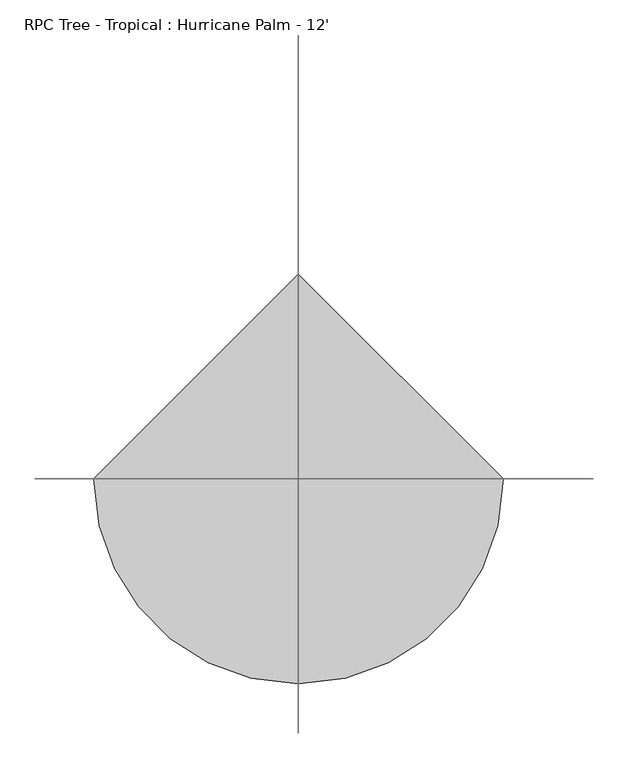
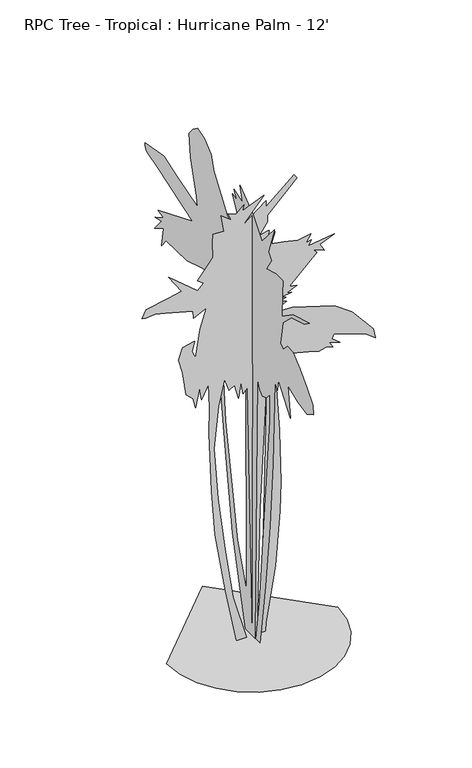
"""IFC4 building model written with IfcOpenShell, lengths in millimetres: geographic element geometry, RPC Tree - Tropical : Hurricane Palm - 12'."""

from ifc_helpers import new_model, si_unit, origin, place, context, project, spatial, triangles, source, transform, mapped, element, save


def rpc_tree_tropical_hurricane_palm_12_75f24be5(model_context):
    return source(origin(), model_context, "Body", "Tessellation", [
        triangles([(-654.0698874, 0.0, 0.0), (-636.7800997, -149.8698129, 0.0), (-587.5320883, -287.499875, 0.0), (-510.2755031, -408.9498928, 0.0), (-408.9498928, -510.2755031, 0.0), (-287.499875, -587.5320883, 0.0), (-149.8695585, -636.7800997, 0.0), (2.86e-05, -654.0698874, 0.0), (149.8698129, -636.7800997, 0.0), (287.499875, -587.5320883, 0.0), (408.9498928, -510.2755031, 0.0), (510.2755031, -408.9498928, 0.0), (587.5320883, -287.499875, 0.0), (636.7800997, -149.8695585, 0.0), (654.0698874, 5.72e-05, 0.0), (-8.58e-05, 654.0698874, 0.0), (318.8205832, -0.0001055, 3607.7882149), (342.0361719, -9.81e-05, 3572.9650497), (117.6189471, -7.01e-05, 3352.4168839), (117.6189471, -6.04e-05, 3298.2640846), (55.7107982, -4.76e-05, 3209.2625404), (129.2264781, -4.66e-05, 3224.731073), (125.3575554, -3.85e-05, 3178.2998955), (175.6579009, -3.94e-05, 3197.6548187), (148.5728899, -2.49e-05, 3108.6532745), (241.4349724, -1.74e-05, 3093.184742), (349.7755614, -7.1e-06, 3066.108197), (450.3747262, -5.5e-06, 3085.4375404), (411.6829382, 2.9e-06, 3027.3986412), (454.2431674, 3.7e-06, 3035.1455521), (431.0301221, 9.5e-06, 2996.4615761), (628.3600468, 1.46e-05, 3023.5378304), (516.1530876, 1.72e-05, 2977.1066528), (550.9764344, 3.01e-05, 2915.2069427), (465.8534689, 1.95e-05, 2950.0303986), (492.9374989, 2.64e-05, 2919.0677536), (283.9972182, 5.18e-05, 2717.874511), (342.0361719, 5.68e-05, 2706.2667892), (264.6500525, 5.85e-05, 2675.3041443), (299.4734356, 6.16e-05, 2667.5825226), (225.9582644, 6e-05, 2655.9748009), (256.9132246, 6.43e-05, 2640.4806885), (206.6115892, 6.45e-05, 2625.0121559), (260.7816294, 7.07e-05, 2605.6572327), (140.8345268, 7.5e-05, 2547.6183334), (307.2127888, 8.41e-05, 2543.7575226), (628.3600468, 0.0001184, 2443.1531982), (759.9166969, 0.0001423, 2346.42262), (926.2942595, 0.0001854, 2152.9585567), (941.7704224, 0.0002007, 2071.7039234), (875.9946407, 0.0001877, 2125.8744541), (624.4916056, 0.0001583, 2218.7368092), (609.0154063, 0.0001638, 2183.9134987), (670.9227831, 0.0001759, 2133.6113365), (589.6682588, 0.0001676, 2156.8269253), (616.7522524, 0.0001766, 2114.2667324), (562.5842288, 0.0001711, 2129.742968), (508.4136981, 0.0001704, 2118.1351009), (431.0301221, 0.0001631, 2137.4823212), (299.4734356, 0.0001502, 2172.3056316), (167.9192925, 0.0001345, 2222.605323), (206.6115892, 0.0002513, 1580.3081909), (218.219638, 0.0003259, 1166.2961071), (210.4810297, 0.0003671, 934.1402922), (179.5268326, 0.000443, 500.7835316), (106.0108984, 0.0005161, 71.2967382), (102.1417123, 0.0005293, 0.0040964), (55.7107982, 0.0005275, 6.75e-05), (86.664741, 0.0003795, 829.6726862), (117.6189471, 0.0001437, 2156.8269253), (59.5799798, 0.0003463, 1007.6579704), (36.3641412, 0.0005257, 0.0040988), (1.5408621, 0.0005239, 0.0041002), (-37.1515409, 0.0001615, 2013.6650242), (-71.9749172, 0.0001667, 1974.9731998), (-87.4518931, 0.0001479, 2075.5724373), (-102.9291188, 0.0001692, 1951.7576111), (-133.8833159, 0.0001469, 2067.8355549), (-176.4450439, 0.0001496, 2040.7489815), (-211.2684271, 0.0001299, 2141.3506897), (-257.700622, 0.0001635, 1940.1498894), (-292.5214617, 0.0002205, 1611.2632782), (-261.5690269, 0.0002961, 1197.2511217), (-207.3989867, 0.000375, 771.6337143), (-145.490856, 0.0004514, 361.4900353), (-44.8901515, 0.0005207, 0.0081326), (-118.4060902, 0.0005178, 0.0041047), (-203.5298188, 0.0004368, 427.2683604), (-284.7846156, 0.0003455, 914.7956881), (-311.8686092, 0.0002797, 1274.6371685), (-331.2157931, 0.000195, 1742.8173122), (-327.3448448, 0.0001579, 1951.7576111), (-335.084198, 0.0001229, 2145.2190582), (-385.3837804, 0.0001397, 2036.8806129), (-400.8625594, 0.000121, 2137.4823212), (-431.8175014, 0.0001457, 1990.4494354), (-451.1621418, 0.0001309, 2067.8355549), (-505.3326725, 0.0001191, 2118.1351009), (-532.4166661, 8.39e-05, 2307.7281796), (-563.3716444, 6.22e-05, 2419.9377548), (-532.4166661, 4.79e-05, 2508.9291252), (-439.5543474, 4.91e-05, 2528.2762001), (-458.901495, 6.2e-05, 2450.890226), (-431.8175014, 7.37e-05, 2392.8537975), (-396.9915748, 3.67e-05, 2609.5180435), (-350.5604336, 1.07e-05, 2768.1664993), (-447.2937006, 1.48e-05, 2717.874511), (-451.1621418, 4.2e-06, 2775.9134102), (-663.9708092, -1.69e-05, 2833.9523094), (-741.3569286, -2.43e-05, 2853.2816528), (-814.8721361, -2.66e-05, 2845.5603218), (-841.9586369, -2.94e-05, 2853.2816528), (-811.0036949, -3.82e-05, 2911.3208427), (-640.7552204, -3.58e-05, 2946.1440079), (-540.1560556, -3.49e-05, 2969.359742), (-640.7552204, -6.62e-05, 3116.4001854), (-416.3387587, -2.1e-05, 2926.8146645), (-373.775986, -2.71e-05, 2973.245842), (-416.3387587, -3.55e-05, 3008.0692978), (-342.8235875, -4.91e-05, 3104.7924637), (-300.260833, -5.66e-05, 3158.9705521), (-304.1317813, -7.76e-05, 3275.0486412), (-300.260833, -8.98e-05, 3344.6952621), (-215.1373588, -8.41e-05, 3336.9483513), (-238.3532019, -0.0001095, 3472.381073), (-160.9678273, -9.45e-05, 3410.4557831), (-184.1836704, -0.0001061, 3468.4946823), (-122.2752672, -9.81e-05, 3441.418428), (-64.2365587, -0.0001056, 3499.4573273), (-75.8440988, -9.78e-05, 3453.0261497), (90.5341814, -0.0001019, 3522.6730614), (-75.8440988, -7.64e-05, 3333.0875404), (106.0108984, -9.21e-05, 3472.381073), (106.0108984, -8.31e-05, 3422.0635048), (3.6e-06, 111.5414929, 2091.8410664), (2.7e-06, 138.6039035, 2014.5184605), (-9.1e-06, 181.1303321, 2238.7520119), (-1.55e-05, 212.059131, 2331.5355927), (-1.87e-05, 258.4524475, 2254.2156029), (-2.47e-05, 328.0408052, 2176.8928516), (-3.28e-05, 405.3634111, 2138.2341648), (-7.8e-06, 351.2385899, 1515.797303), (3.68e-05, 192.7289882, 653.6635168), (6.06e-05, 76.7468144, 317.3169322), (5e-06, 84.4790731, 2153.6976105), (-2.35e-05, 722.380616, 3657.5976746), (-1.2e-05, 633.4603895, 3626.6606094), (8e-07, 544.5400904, 3553.203756), (8.1e-06, 509.7471923, 3448.8351265), (2.39e-05, 413.0951703, 3305.7825211), (3.76e-05, 328.0408052, 3185.945359), (4.85e-05, 246.8535552, 3143.4002815), (5.72e-05, 157.9343097, 3209.1355133), (3.88e-05, 262.318327, 3406.3156288), (4.67e-05, 200.4607292, 3390.8470963), (3.98e-05, 242.9874212, 3452.6959373), (5.46e-05, 127.0055108, 3417.8980614), (4.69e-05, 161.799935, 3537.7605125), (7.16e-05, -12.1727138, 3406.3156288), (8.98e-05, -128.1548593, 3259.4022125), (0.0001038, -294.3959657, 3452.6959373), (0.0001008, -213.2082251, 3228.4648567), (0.0001074, -255.7346628, 3178.1984482), (0.0001022, -186.1458145, 3073.8298187), (0.0001164, -313.7253636, 3108.6276947), (0.0001274, -406.5114879, 3108.6276947), (0.0001299, -398.7797287, 2996.5121544), (0.0001348, -394.9138673, 2814.8008621), (0.0001489, -537.9589514, 2915.30839), (0.0001728, -754.4582365, 2977.1575218), (0.0001669, -692.6016924, 2930.7772133), (0.0001481, -522.4928896, 2880.5105141), (0.0001375, -406.5114879, 2772.2557846), (0.000139, -371.7160463, 2582.8228706), (0.0001443, -410.3773856, 2559.6324257), (0.000149, -464.5022069, 2617.6207466), (0.0001579, -537.9589514, 2613.7599358), (0.0001717, -634.6084299, 2536.4373299), (0.0001852, -723.5287291, 2439.787706), (0.0001976, -804.7172327, 2347.0016544), (0.0002007, -812.4489555, 2273.5449463), (0.0001916, -723.5287291, 2223.2859501), (0.0001765, -603.6814296, 2250.3497051), (0.0001597, -476.0998275, 2304.4744537), (0.0001703, -503.1635098, 2057.0456612), (0.0001455, -348.5208052, 2269.6790485), (0.0001463, -333.0572868, 2180.7613655), (0.0001413, -302.1277249, 2227.1518478), (0.0001582, -275.0640425, 1550.5902374), (0.0001693, -236.4045018, 1024.8055429), (0.0001778, -178.4135466, 506.752535), (0.0001841, -104.9583191, 0.0066211), (0.0001776, -50.8332435, 0.0066227), (0.0001732, -93.3601808, 321.1827936), (0.0001439, -236.4045018, 1875.3417812), (0.0001376, -236.4045018, 2087.9751686), (0.0001337, -190.011694, 2033.85042), (0.0001278, -135.8868637, 2014.5184605), (0.0001228, -101.0921852, 2041.5820702), (0.000117, -70.1636452, 2115.0363075), (0.0001762, -39.2348462, 0.0106537), (0.0001612, 88.3452071, 0.0066269), (0.0001208, 258.4524475, 672.9928602), (8.92e-05, 362.8362104, 1314.7616089), (5.46e-05, 463.3541302, 2072.5091068), (5.04e-05, 463.3541302, 2215.5541546), (4.58e-05, 513.6130537, 2169.1612015), (4.52e-05, 467.2199916, 2374.0627934), (3.97e-05, 509.7471923, 2389.5288551), (3.84e-05, 486.5493713, 2524.839782), (3.4e-05, 529.076572, 2501.6443954), (2.95e-05, 544.5400904, 2590.5697815), (1.56e-05, 668.2557947, 2563.4932365), (-5.6e-06, 861.5572952, 2501.6443954), (-3.86e-05, 1139.9157406, 2493.9125999), (-4.33e-05, 1197.9063869, 2420.4558918), (-4.46e-05, 1170.8427046, 2571.2404381), (-5.69e-05, 1290.6925838, 2505.5101479), (-4.92e-05, 1197.9063869, 2617.6207466), (-5.87e-05, 1282.9607883, 2598.2914032), (-4.77e-05, 1174.7111458, 2660.1402443), (-5.66e-05, 1244.2994854, 2679.4951675), (-8.2e-06, 791.9689556, 2865.0419815), (-6.51e-05, 1232.7017921, 3011.9553978), (-8.63e-05, 1398.9422264, 3058.3612862), (-8.96e-05, 1418.2715698, 3093.1591621), (-9.03e-05, 1418.2715698, 3116.3493164), (-6.16e-05, 1166.9768795, 3158.8691048), (-3.82e-05, 985.2729996, 3100.8807838), (-4.9e-06, 726.2465137, 3019.7025993), (-8.3e-06, 733.9782366, 3100.8807838), (-2.59e-05, 815.1667402, 3367.6313622), (-3.36e-05, 834.4961563, 3549.3429451), (-2.95e-05, 784.2372328, 3611.217366), (4.94e-05, 30.3542496, 2215.5541546), (0.0001139, 3.2915585, 158.8072942), (5.52e-05, -12.1726377, 2192.3589134)], [[15, 16, 1], [14, 15, 1], [14, 1, 2], [13, 14, 2], [13, 2, 3], [13, 3, 4], [12, 13, 4], [11, 12, 4], [11, 4, 5], [11, 5, 6], [11, 6, 7], [11, 7, 8], [11, 8, 9], [11, 9, 10], [31, 32, 33], [115, 116, 117], [39, 40, 41], [76, 77, 78], [53, 54, 55], [95, 96, 97], [130, 131, 132], [128, 129, 130], [37, 38, 39], [93, 94, 95], [33, 34, 35], [49, 50, 51], [31, 33, 35], [55, 56, 57], [124, 125, 126], [41, 42, 43], [126, 127, 128], [27, 28, 29], [43, 44, 45], [29, 30, 31], [74, 75, 76], [23, 24, 25], [132, 133, 134], [101, 102, 103], [106, 107, 108], [100, 101, 103], [21, 22, 23], [128, 130, 132], [126, 128, 132], [78, 79, 80], [85, 86, 87], [85, 87, 88], [84, 85, 88], [84, 88, 89], [83, 84, 89], [83, 89, 90], [82, 83, 90], [82, 90, 91], [81, 82, 91], [81, 91, 92], [48, 49, 51], [48, 51, 52], [111, 112, 113], [47, 48, 52], [110, 111, 113], [110, 113, 114], [109, 110, 114], [134, 17, 18], [134, 18, 19], [132, 134, 19], [95, 97, 98], [67, 68, 69], [66, 67, 69], [65, 66, 69], [64, 65, 69], [64, 69, 70], [63, 64, 70], [62, 63, 70], [61, 62, 70], [124, 126, 132], [132, 19, 20], [132, 20, 21], [95, 98, 99], [122, 123, 124], [99, 100, 103], [99, 103, 104], [72, 73, 74], [71, 72, 74], [70, 71, 74], [70, 74, 76], [118, 119, 120], [95, 99, 104], [93, 95, 104], [35, 36, 37], [80, 81, 92], [80, 92, 93], [108, 109, 114], [108, 114, 115], [108, 115, 117], [106, 108, 117], [31, 35, 37], [46, 47, 52], [46, 52, 53], [46, 53, 55], [46, 55, 57], [46, 57, 58], [46, 58, 59], [46, 59, 60], [46, 60, 61], [45, 46, 61], [80, 93, 104], [106, 117, 118], [29, 31, 37], [27, 29, 37], [26, 27, 37], [25, 26, 37], [121, 122, 124], [121, 124, 132], [121, 132, 21], [76, 78, 80], [80, 104, 105], [70, 76, 80], [70, 80, 105], [61, 70, 105], [45, 61, 105], [45, 105, 106], [43, 45, 106], [41, 43, 106], [41, 106, 118], [41, 118, 120], [41, 120, 121], [41, 121, 21], [41, 21, 23], [41, 23, 25], [41, 25, 37], [41, 37, 39], [235, 144, 145], [144, 235, 236], [219, 220, 221], [160, 161, 162], [169, 170, 171], [169, 171, 172], [217, 218, 219], [215, 216, 217], [184, 185, 186], [135, 136, 137], [168, 169, 172], [168, 172, 173], [206, 207, 208], [157, 158, 159], [221, 222, 223], [155, 156, 157], [186, 187, 188], [145, 135, 146], [145, 146, 147], [145, 147, 148], [145, 148, 149], [145, 149, 150], [145, 150, 151], [153, 154, 155], [145, 151, 152], [235, 145, 152], [210, 211, 212], [192, 193, 194], [191, 192, 194], [191, 194, 195], [190, 191, 195], [189, 190, 195], [188, 189, 195], [188, 195, 196], [165, 166, 167], [153, 155, 157], [153, 157, 159], [153, 159, 160], [226, 227, 228], [225, 226, 228], [224, 225, 228], [223, 224, 228], [223, 228, 229], [223, 229, 230], [208, 209, 210], [201, 202, 203], [162, 163, 164], [160, 162, 164], [153, 160, 164], [214, 215, 217], [164, 165, 167], [164, 167, 168], [235, 152, 153], [235, 153, 164], [235, 164, 168], [235, 168, 173], [235, 173, 174], [237, 235, 174], [237, 174, 175], [180, 181, 182], [179, 180, 182], [179, 182, 183], [179, 183, 184], [178, 179, 184], [177, 178, 184], [176, 177, 184], [175, 176, 184], [237, 175, 184], [237, 184, 186], [237, 186, 188], [237, 188, 196], [237, 196, 197], [217, 219, 221], [214, 217, 221], [214, 221, 223], [213, 214, 223], [212, 213, 223], [212, 223, 230], [197, 198, 199], [197, 199, 200], [237, 197, 200], [236, 237, 200], [236, 200, 201], [236, 201, 203], [144, 236, 203], [143, 144, 203], [142, 143, 203], [142, 203, 204], [142, 204, 205], [141, 142, 205], [141, 205, 206], [140, 141, 206], [140, 206, 208], [139, 140, 208], [138, 139, 208], [138, 208, 210], [232, 233, 234], [232, 234, 146], [231, 232, 146], [210, 212, 230], [138, 210, 230], [138, 230, 231], [138, 231, 146], [138, 146, 135], [138, 135, 137]], closed=False),
    ])


if __name__ == "__main__":
    model = new_model("IFC4")
    model_context = context("Model", 3, world=origin())
    ifc_project = project(units=[si_unit("LENGTHUNIT", "METRE", prefix="MILLI")], contexts=[model_context])
    site = spatial("IfcSite", under=ifc_project)
    building = spatial("IfcBuilding", under=site)
    placement = place(None, origin())
    rpc_tree_tropical_hurricane_palm_12_shape = rpc_tree_tropical_hurricane_palm_12_75f24be5(model_context)
    element("IfcGeographicElement", 1, ObjectType="RPC Tree - Tropical : Hurricane Palm - 12'", at=placement, inside=building, context=model_context, shape_type="MappedRepresentation", body=[
        mapped(rpc_tree_tropical_hurricane_palm_12_shape, transform((0.0, 0.0, 0.0), x_axis=(1.0, 0.0, 0.0), y_axis=(0.0, 1.0, 0.0), z_axis=(0.0, 0.0, 1.0))),
    ])
    save(model, "model.ifc")

# Revit data of these elements
# Type "RPC Tree - Tropical : Hurricane Palm - 12'"
#   built-in parameter 1005198 = "{2, 15},{39, RPC-16-FXGL-UL7X-PH44-0000-ST1L-LVER-AU},{1, 0},{1, 0},{2, 13},{1, 8},{5, Color},{1, 0},{1, 0},{3, 0.8},{3, 0.8},{3, 0.8},{1, 8},{7, BBoxMin},{1, 0},{1, 0},{1, 0},{1, 0},{1, 0},{1, 8},{7, BBoxMax},{1, 0},{1, 0},{1, 0},{1, 0},{1, 0},{2, 11},{9, RPCTypeId},{1, 0},{1, 0},{39, RPC-16-FXGL-UL7X-PH44-0000-ST1L-LVER-AU},{1, 6},{14, RPCPlantHeight},{1, 0},{1, 0},{2, 12},{2, 11},{7, keyword},{1, 0},{1, 0},{35, :RPCs:Trees [Tropical]:Geometry:RPC},{2, 11},{8, category},{1, 0},{1, 0},{16, Trees [Tropical]},{2, 11},{12, LocalizedUID},{1, 0},{1, 0},{14, Hurricane Palm},{2, 14},{6, Height},{1, 0},{1, 0},{2, 12},{1, 2},{16, Cast Reflections},{1, 0},{1, 0},{1, 0},{1, 2},{12, Cast Shadows},{1, 0},{1, 0},{1, 1},{1, 2},{9, Lock View},{1, 0},{1, 0},{1, 0},{1, 4},{5, ViewC},{1, 0},{1, 0},{1, 0},{21, assetlibrary_base.fbx},{1, 5},"
#   built-in parameter 1005195 = "RPC-16-FXGL-UL7X-PH44-0000-ST1L-LVER-AU"
#   Type Comments = "Hurricane Palm"
#   Assembly Code = "G2050500"
#   Height = 12' - 0"
#   Plan Symbol = element 387627
#   Default Elevation = 0
